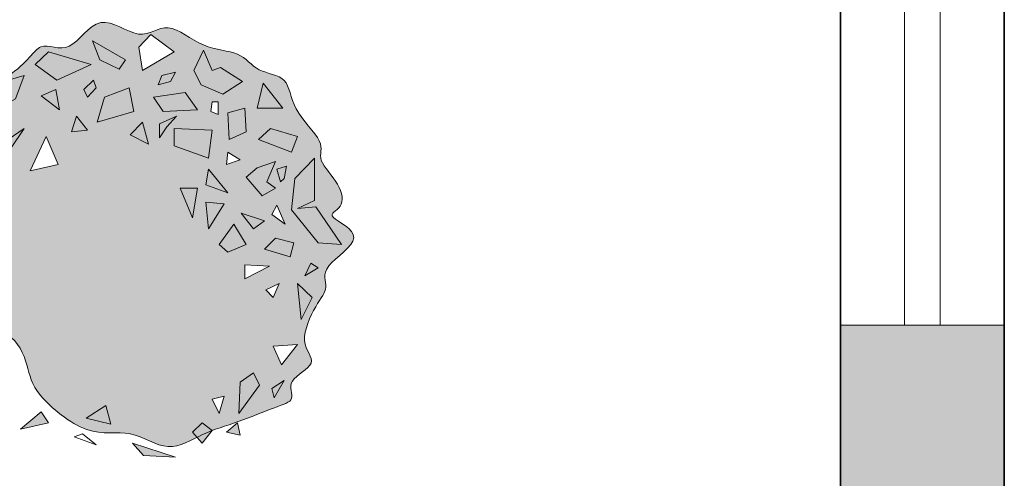
# Model space of a CAD drawing. Units: metres. Extents: x 4298.5 to 4325.2, y 2075 to 2095.8.
# Tile 14 of 35: x 4304.508 to 4305.891, y 2083.045 to 2083.689. Entities that reach past the tile are written whole.
import ezdxf

# ---------------------------------------------------------------- set-up
doc = ezdxf.new("R2010")
doc.units = ezdxf.units.M
for name, color, linetype, lineweight in [('A-ANNO-DIMS', 2, 'Continuous', 18), ('A-GLAZ', 4, 'Continuous', 18), ('A-WALL', 7, 'Continuous', 35), ('A-WALL-PATT', 252, 'Continuous', 13), ('L-PLNT', 94, 'Continuous', 13)]:
    doc.layers.add(name, color=color, linetype=linetype, lineweight=lineweight)
doc.layers.add('L-PLNT-PATT', color=116, linetype='Continuous', lineweight=13, true_color=0x13823e)
doc.styles.get("Standard").update_dxf_attribs({"font": 'arial.ttf'})
doc.dimstyles.get("Standard").update_dxf_attribs({"dimtxt": 0.18, "dimasz": 0.18, "dimexe": 0.18, "dimexo": 0.0625, "dimgap": 0.09, "dimtad": 0, "dimtih": 1, "dimtoh": 1, "dimdec": 4, "dimzin": 0, "dimdsep": 46, "dimtxsty": 'Standard', "dimcen": 0.09, "dimadec": 0, "dimazin": 0, "dimtfac": 1, "dimtdec": 4, "dimtofl": 0, "dimtmove": 0, "dimatfit": 3, "dimfxl": 1, "dimtolj": 1, "dimtzin": 0, "dimarcsym": 0})

# ---------------------------------------------------------------- blocks, each defined once
blk = doc.blocks.new('*U9')
for points in [[(1.237, 12.003), (0.562, 11.31), (0.764, 10.013), (2.519, 11.051)], [(-2.003, 11.656), (-1.598, 10.618), (-0.518, 10.099), (-0.181, 10.618), (-0.788, 10.964)], [(-4.432, 11.051), (-5.175, 10.359), (-3.96, 9.493), (-2.07, 10.359)], [(4.139, 11.137), (3.599, 10.013), (4.004, 9.234), (5.218, 8.715), (6.298, 9.407), (5.083, 10.186), (4.611, 10.013)], [(2.586, 9.926), (1.844, 9.753), (1.642, 9.234), (2.316, 9.407)], [(-5.782, 9.753), (-7.537, 9.234), (-8.009, 7.504), (-6.255, 8.455)], [(-1.935, 9.493), (-2.475, 8.974), (-2.273, 8.542), (-1.8, 9.061)], [(7.446, 9.32), (7.108, 7.936), (8.525, 7.936)], [(-4.837, 8.628), (-3.825, 7.85), (-4.027, 8.974)], [(0.022, 9.061), (-1.328, 8.542), (-1.733, 7.157), (0.292, 7.763)], [(1.372, 8.542), (3.126, 8.801), (3.801, 7.85), (1.912, 7.763)], [(4.611, 8.282), (4.544, 7.763), (4.949, 7.59), (4.949, 8.282)], [(6.433, 7.936), (5.488, 7.676), (5.556, 6.206), (6.501, 6.638)], [(-2.88, 7.504), (-3.15, 6.638), (-2.273, 6.725)], [(0.764, 7.157), (0.089, 6.465), (1.102, 5.946)], [(1.709, 6.292), (1.709, 7.071), (2.654, 7.504), (2.114, 6.898)], [(-5.782, 6.811), (-6.659, 6.206), (-6.524, 5.687)], [(2.519, 6.811), (2.519, 5.86), (4.409, 5.167), (4.611, 6.725)], [(7.851, 6.811), (7.176, 6.206), (8.998, 5.514), (9.335, 6.379)], [(-8.144, 6.033), (-9.359, 5.946), (-9.022, 4.735)], [(-4.567, 6.379), (-5.445, 4.475), (-3.892, 4.821)], [(5.488, 5.514), (5.421, 4.821), (6.163, 5.081)], [(8.12, 4.994), (7.108, 4.648), (6.501, 4.129), (7.378, 3.091), (8.12, 3.524), (7.648, 3.87)], [(10.28, 5.167), (9.2, 4.043), (8.998, 2.312), (10.482, 0.495), (11.765, 0.409), (10.348, 2.485), (9.335, 2.399), (10.28, 2.831)], [(4.409, 4.562), (4.274, 3.697), (5.488, 3.264)], [(8.728, 4.735), (8.188, 4.562), (8.39, 3.87), (8.593, 4.043)], [(-11.316, 1.793), (-9.831, 2.312), (-9.629, 3.437), (-10.439, 3.524)], [(3.531, 1.88), (2.856, 3.524), (3.801, 3.524)], [(-8.212, 3.091), (-8.482, 2.312), (-7.874, 2.572)], [(4.274, 2.745), (5.286, 2.658), (4.409, 1.274)], [(8.188, 2.572), (7.918, 2.053), (8.66, 1.534)], [(-6.997, 1.793), (-7.942, 1.534), (-7.469, 0.495)], [(7.513, 1.707), (6.906, 1.274), (6.231, 2.139)], [(5.826, 1.534), (5.016, 0.409), (5.488, -0.024), (6.501, 0.409)], [(-8.212, 0.409), (-9.426, 0.322), (-9.831, 0.841)], [(8.12, 0.755), (7.513, 0.149), (8.93, -0.283), (9.133, 0.495)], [(7.783, -0.803), (6.433, -1.495), (6.433, -0.716)], [(10.078, -0.629), (9.74, -1.322), (10.482, -0.889)], [(8.323, -1.754), (7.985, -2.533), (7.581, -2.1)], [(9.335, -1.754), (9.538, -3.744), (10.145, -2.533)], [(-10.034, -2.706), (-10.641, -3.312), (-10.439, -4.436), (-9.899, -3.485)], [(-8.279, -5.734), (-6.794, -5.302), (-6.997, -6.513)], [(9.335, -5.129), (8.458, -6.253), (7.985, -5.215)], [(6.096, -8.935), (6.163, -7.205), (6.906, -6.686), (7.243, -7.378)], [(8.053, -8.07), (8.593, -7.118), (7.918, -7.551)], [(5.286, -7.984), (4.611, -8.157), (5.016, -8.935)], [(-2.34, -9.195), (-1.26, -8.503), (-0.99, -9.541)], [(-4.837, -8.849), (-4.432, -9.454), (-5.985, -9.801)], [(4.071, -9.454), (3.531, -9.974), (4.071, -10.579), (4.611, -9.887)], [(6.028, -9.454), (5.421, -9.974), (6.163, -10.147)], [(-2.543, -10.06), (-3.015, -10.233), (-1.8, -10.666)], [(0.224, -10.579), (0.832, -11.272), (2.586, -11.358)]]:
    blk.add_lwpolyline(points, close=True)
blk = doc.blocks.new('WIN-760-GLASS')
for p, q in [((0, 0.76), (0, 0)), ((0.05, 0.76), (0.05, 0))]:
    blk.add_line(p, q)
blk = doc.blocks.new('*D47')
at = {"layer": 'A-ANNO-DIMS', "color": 0, "lineweight": -2, "transparency": 16777216}
for p, q in [((4300.4306, 2084.4956), (4300.4306, 2074.9896)), ((4322.8106, 2084.4956), (4322.8106, 2074.9896)), ((4300.6106, 2075.1696), (4311.2252, 2075.1696)), ((4322.6306, 2075.1696), (4312.016, 2075.1696))]:
    blk.add_line(p, q, dxfattribs=at)
at = {"layer": 'A-ANNO-DIMS', "color": 0, "transparency": 16777216}
for points in [[(4300.6106, 2075.1996), (4300.6106, 2075.1396), (4300.4306, 2075.1696)], [(4322.6306, 2075.1996), (4322.6306, 2075.1396), (4322.8106, 2075.1696)]]:
    blk.add_solid(points, dxfattribs=at)
at = {"layer": 'Defpoints', "color": 0, "transparency": 16777216}
for p in [(4300.4306, 2084.5581), (4322.8106, 2084.5581), (4322.8106, 2075.1696)]:
    blk.add_point(p, dxfattribs=at)
at = {"layer": 'A-ANNO-DIMS', "color": 0, "transparency": 16777216, "insert": (4311.6206, 2075.1696), "char_height": 0.18, "attachment_point": 5}
blk.add_mtext('\\A1;22.38', dxfattribs=at)
blk = doc.blocks.new('*D51')
at = {"layer": 'A-ANNO-DIMS', "color": 0, "lineweight": -2, "transparency": 16777216}
for p, q in [((4305.5981, 2084.5581), (4299.0921, 2084.5581)), ((4299.2721, 2084.3781), (4299.2721, 2082.375)), ((4299.2721, 2080.0081), (4299.2721, 2082.0111)), ((4305.5981, 2079.8281), (4299.0921, 2079.8281))]:
    blk.add_line(p, q, dxfattribs=at)
at = {"layer": 'A-ANNO-DIMS', "color": 0, "transparency": 16777216}
for points in [[(4299.2421, 2084.3781), (4299.3021, 2084.3781), (4299.2721, 2084.5581)], [(4299.2421, 2080.0081), (4299.3021, 2080.0081), (4299.2721, 2079.8281)]]:
    blk.add_solid(points, dxfattribs=at)
at = {"layer": 'Defpoints', "color": 0, "transparency": 16777216}
for p in [(4305.6606, 2084.5581), (4299.2721, 2079.8281), (4305.6606, 2079.8281)]:
    blk.add_point(p, dxfattribs=at)
at = {"layer": 'A-ANNO-DIMS', "color": 0, "transparency": 16777216, "insert": (4299.2721, 2082.1931), "char_height": 0.18, "attachment_point": 5}
blk.add_mtext('\\A1;4.73', dxfattribs=at)
blk = doc.blocks.new('*D56')
at = {"layer": 'A-ANNO-DIMS', "color": 0, "lineweight": -2, "transparency": 16777216}
for p, q in [((4305.8281, 2085.0581), (4299.0921, 2085.0581)), ((4299.2721, 2084.8781), (4299.2721, 2083.74)), ((4299.2721, 2082.2381), (4299.2721, 2083.3761)), ((4305.8281, 2082.0581), (4299.0921, 2082.0581))]:
    blk.add_line(p, q, dxfattribs=at)
at = {"layer": 'A-ANNO-DIMS', "color": 0, "transparency": 16777216}
for points in [[(4299.2421, 2084.8781), (4299.3021, 2084.8781), (4299.2721, 2085.0581)], [(4299.2421, 2082.2381), (4299.3021, 2082.2381), (4299.2721, 2082.0581)]]:
    blk.add_solid(points, dxfattribs=at)
at = {"layer": 'Defpoints', "color": 0, "transparency": 16777216}
for p in [(4299.2721, 2085.0581), (4305.8906, 2085.0581), (4305.8906, 2082.0581)]:
    blk.add_point(p, dxfattribs=at)
at = {"layer": 'A-ANNO-DIMS', "color": 0, "transparency": 16777216, "insert": (4299.2721, 2083.5581), "char_height": 0.18, "attachment_point": 5}
blk.add_mtext('\\A1;3', dxfattribs=at)

msp = doc.modelspace()

# ---------------------------------------------------------------- hatches: boundary and pattern name
at = {"layer": 'A-WALL-PATT'}
h = msp.add_hatch(color=256, dxfattribs=at)
h.dxf.hatch_style = 1
h.paths.add_polyline_path([(4308.7606, 2094.4781), (4308.1606, 2094.4781), (4307.4606, 2094.4781), (4307.4606, 2094.2481), (4308.2706, 2094.2481), (4308.2706, 2094.1281), (4308.3906, 2094.1281), (4308.3906, 2094.2481), (4308.7606, 2094.2481)])
h.paths.add_polyline_path([(4310.1206, 2094.4781), (4309.5206, 2094.4781), (4309.5206, 2094.2481), (4309.8906, 2094.2481), (4309.8906, 2092.2481), (4308.3906, 2092.2481), (4308.3906, 2093.4281), (4308.2706, 2093.4281), (4308.2706, 2092.0181), (4309.8906, 2092.0181), (4309.8906, 2087.0181), (4309.7706, 2087.0181), (4309.7706, 2086.7881), (4309.8906, 2086.7881), (4311.9406, 2086.7881), (4311.9406, 2087.0181), (4310.1206, 2087.0181), (4310.1206, 2089.0181), (4310.2406, 2089.0181), (4310.2406, 2089.1381), (4310.1206, 2089.1381), (4310.1206, 2092.0181), (4310.3078, 2092.0181), (4310.3078, 2092.2481), (4310.1206, 2092.2481)])
h.paths.add_polyline_path([(4311.7406, 2092.2481), (4311.0678, 2092.2481), (4311.0678, 2092.0181), (4311.7406, 2092.0181)], flags=17)
h.paths.add_polyline_path([(4313.1733, 2092.2481), (4312.5006, 2092.2481), (4312.5006, 2092.0181), (4313.1733, 2092.0181)])
h.paths.add_polyline_path([(4314.5378, 2092.2481), (4314.1206, 2092.2481), (4313.9333, 2092.2481), (4313.9333, 2092.0181), (4314.1206, 2092.0181), (4314.1206, 2087.0181), (4314.0006, 2087.0181), (4314.0006, 2086.7881), (4314.1206, 2086.7881), (4315.5718, 2086.7881), (4315.5718, 2087.0181), (4314.3506, 2087.0181), (4314.3506, 2092.0181), (4314.5378, 2092.0181)])
h.paths.add_polyline_path([(4315.9706, 2092.2481), (4315.2978, 2092.2481), (4315.2978, 2092.0181), (4315.9706, 2092.0181)])
h.paths.add_polyline_path([(4317.4033, 2092.2481), (4316.7306, 2092.2481), (4316.7306, 2092.0181), (4317.4033, 2092.0181)])
h.paths.add_polyline_path([(4318.9506, 2092.2481), (4318.3506, 2092.2481), (4318.1633, 2092.2481), (4318.1633, 2092.0181), (4318.3506, 2092.0181), (4318.3506, 2091.8981), (4318.5806, 2091.8981), (4318.5806, 2092.0181), (4318.9506, 2092.0181)])
h.paths.add_polyline_path([(4321.0106, 2092.2481), (4319.7106, 2092.2481), (4319.7106, 2092.0181), (4320.0806, 2092.0181), (4320.0806, 2090.0181), (4318.5806, 2090.0181), (4318.5806, 2091.1981), (4318.3506, 2091.1981), (4318.3506, 2090.0181), (4318.3506, 2087.0181), (4318.2306, 2087.0181), (4318.2306, 2086.7881), (4318.3506, 2086.7881), (4318.3506, 2086.3081), (4318.5806, 2086.3081), (4318.5806, 2089.7881), (4321.7806, 2089.7881), (4321.7806, 2090.0181), (4320.2006, 2090.0181), (4320.2006, 2092.0181), (4321.0106, 2092.0181)])
h.paths.add_polyline_path([(4322.8106, 2092.2481), (4321.7706, 2092.2481), (4321.7706, 2092.0181), (4322.5806, 2092.0181), (4322.5806, 2091.2831), (4322.8106, 2091.2831)])
h.paths.add_polyline_path([(4322.8106, 2090.5231), (4322.5806, 2090.5231), (4322.5806, 2089.7881), (4322.5806, 2089.5254), (4322.8106, 2089.5254), (4322.8106, 2090.0181)])
h.paths.add_polyline_path([(4322.8106, 2088.7654), (4322.5806, 2088.7654), (4322.5806, 2087.6681), (4322.8106, 2087.6681)])
h.paths.add_polyline_path([(4322.8106, 2086.9081), (4322.5806, 2086.9081), (4322.5806, 2085.8107), (4322.8106, 2085.8107)])
h.paths.add_polyline_path([(4322.8106, 2085.0507), (4322.5806, 2085.0507), (4322.5806, 2084.7881), (4318.5806, 2084.7881), (4318.5806, 2085.0581), (4318.5806, 2085.4081), (4318.3506, 2085.4081), (4318.3506, 2084.5581), (4318.3506, 2080.8581), (4318.4706, 2080.8581), (4318.4706, 2082.3281), (4319.2606, 2082.3281), (4319.2606, 2082.5581), (4318.5806, 2082.5581), (4318.5806, 2084.5581), (4320.0806, 2084.5581), (4320.0806, 2083.9381), (4320.3106, 2083.9381), (4320.3106, 2084.5581), (4322.8106, 2084.5581)])
h.paths.add_polyline_path([(4320.3106, 2083.1781), (4320.0806, 2083.1781), (4320.0806, 2082.5581), (4319.9606, 2082.5581), (4319.9606, 2082.3281), (4320.0806, 2082.3281), (4320.0806, 2081.5731), (4320.3106, 2081.5731)], flags=17)
h.paths.add_polyline_path([(4320.3106, 2080.8131), (4320.0806, 2080.8131), (4320.0806, 2080.0581), (4318.4286, 2080.0581), (4318.4286, 2079.8281), (4320.3106, 2079.8281)])
h.paths.add_polyline_path([(4317.3506, 2085.2881), (4316.5718, 2085.2881), (4316.5718, 2085.0581), (4317.3506, 2085.0581)])
h.paths.add_polyline_path([(4315.5718, 2085.2881), (4314.8434, 2085.2881), (4314.8434, 2085.0581), (4315.5718, 2085.0581)])
h.paths.add_polyline_path([(4313.8434, 2085.2881), (4312.9406, 2085.2881), (4312.9406, 2085.0581), (4313.8434, 2085.0581)])
h.paths.add_polyline_path([(4311.9406, 2085.2881), (4311.4406, 2085.2881), (4311.4406, 2085.0581), (4311.9406, 2085.0581)])
h.paths.add_polyline_path([(4317.3306, 2087.0181), (4316.5718, 2087.0181), (4316.5718, 2086.7881), (4317.3306, 2086.7881)])
h.paths.add_polyline_path([(4313.1006, 2089.1381), (4311.1406, 2089.1381), (4311.1406, 2089.0181), (4312.9806, 2089.0181), (4312.9806, 2087.0181), (4312.9406, 2087.0181), (4312.9406, 2086.7881), (4313.1006, 2086.7881), (4313.1006, 2087.0181)])
h.paths.add_polyline_path([(4307.5515, 2087.0181), (4305.8906, 2087.0181), (4305.8906, 2092.2481), (4305.8906, 2094.2481), (4306.7006, 2094.2481), (4306.7006, 2094.4781), (4305.6606, 2094.4781), (4305.6606, 2092.2481), (4305.2906, 2092.2481), (4305.2906, 2092.0181), (4305.6606, 2092.0181), (4305.6606, 2090.0181), (4304.1606, 2090.0181), (4304.1606, 2091.1981), (4304.0406, 2091.1981), (4304.0406, 2089.9081), (4301.5606, 2089.9081), (4301.5606, 2089.7881), (4304.0406, 2089.7881), (4305.6606, 2089.7881), (4305.6606, 2086.6381), (4305.8906, 2086.6381), (4305.8906, 2086.7881), (4307.5515, 2086.7881)])
h.paths.add_polyline_path([(4307.5515, 2085.2881), (4305.8906, 2085.2881), (4305.8906, 2085.4381), (4305.6606, 2085.4381), (4305.6606, 2084.7881), (4305.2906, 2084.7881), (4305.2906, 2084.5581), (4305.6606, 2084.5581), (4305.6606, 2084.02), (4305.8906, 2084.02), (4305.8906, 2084.5581), (4305.8906, 2085.0581), (4307.5515, 2085.0581)])
h.paths.add_polyline_path([(4310.2406, 2085.2881), (4308.5515, 2085.2881), (4308.5515, 2085.0581), (4310.2406, 2085.0581)])
h.paths.add_polyline_path([(4317.4286, 2080.0581), (4316.5718, 2080.0581), (4316.5718, 2079.8281), (4317.4286, 2079.8281)])
h.paths.add_polyline_path([(4315.5718, 2080.0581), (4314.8434, 2080.0581), (4314.8434, 2079.8281), (4315.5718, 2079.8281)])
h.paths.add_polyline_path([(4313.8434, 2080.0581), (4312.9406, 2080.0581), (4312.9406, 2079.8281), (4313.8434, 2079.8281)])
h.paths.add_polyline_path([(4311.9406, 2080.0581), (4311.4406, 2080.0581), (4311.4406, 2079.8281), (4311.9406, 2079.8281)])
h.paths.add_polyline_path([(4310.2406, 2080.0581), (4310.1206, 2080.0581), (4310.1206, 2084.0381), (4309.8906, 2084.0381), (4309.8906, 2080.0581), (4309.1606, 2080.0581), (4309.1606, 2079.8281), (4310.2406, 2079.8281)])
h.paths.add_polyline_path([(4308.1606, 2080.0581), (4307.5106, 2080.0581), (4307.5106, 2080.1781), (4307.3906, 2080.1781), (4307.3906, 2080.0581), (4305.8906, 2080.0581), (4305.8906, 2080.567), (4305.6606, 2080.567), (4305.6606, 2079.8281), (4308.1606, 2079.8281)])
h.paths.add_polyline_path([(4307.5106, 2081.9381), (4309.0906, 2081.9381), (4309.0906, 2082.0581), (4305.8906, 2082.0581), (4305.8906, 2083.26), (4305.6606, 2083.26), (4305.6606, 2081.327), (4305.8906, 2081.327), (4305.8906, 2081.9381), (4307.3906, 2081.9381), (4307.3906, 2080.8781), (4307.5106, 2080.8781)])
h.paths.add_polyline_path([(4304.5306, 2084.7881), (4302.7306, 2084.7881), (4302.7306, 2084.5581), (4304.5306, 2084.5581)])
h.paths.add_polyline_path([(4301.9706, 2084.7881), (4300.6606, 2084.7881), (4300.6606, 2085.0249), (4300.4306, 2085.0249), (4300.4306, 2084.5581), (4301.9706, 2084.5581)])
h.paths.add_polyline_path([(4300.6606, 2086.8843), (4300.4306, 2086.8843), (4300.4306, 2085.7849), (4300.6606, 2085.7849)])
h.paths.add_polyline_path([(4300.6606, 2089.1618), (4300.4306, 2089.1618), (4300.4306, 2087.6443), (4300.6606, 2087.6443)])
h.paths.add_polyline_path([(4300.6606, 2091.0212), (4300.4306, 2091.0212), (4300.4306, 2089.9218), (4300.6606, 2089.9218)])
h.paths.add_polyline_path([(4300.6606, 2092.0181), (4301.9706, 2092.0181), (4301.9706, 2092.2481), (4300.4306, 2092.2481), (4300.4306, 2091.7812), (4300.6606, 2091.7812)])
h.paths.add_polyline_path([(4304.5306, 2092.2481), (4302.7306, 2092.2481), (4302.7306, 2092.0181), (4304.0406, 2092.0181), (4304.0406, 2091.8981), (4304.1606, 2091.8981), (4304.1606, 2092.0181), (4304.5306, 2092.0181)], flags=17)
at = {"layer": 'L-PLNT-PATT'}
h = msp.add_hatch(color=256, dxfattribs=at)
h.dxf.hatch_style = 1
edge = h.paths.add_edge_path()
edge.add_spline(control_points=[(4304.7568, 2083.1024), (4304.7594, 2083.1037), (4304.778, 2083.1131), (4304.8138, 2083.1228), (4304.8683, 2083.1461), (4304.8977, 2083.1537), (4304.8789, 2083.1822), (4304.9315, 2083.2063), (4304.8978, 2083.2327), (4304.9248, 2083.2924), (4304.9435, 2083.3119), (4304.9269, 2083.3404), (4305.0011, 2083.3852), (4304.9312, 2083.4148), (4304.9639, 2083.4224), (4304.9599, 2083.4576), (4304.9218, 2083.4942), (4304.9404, 2083.5135), (4304.8873, 2083.5645), (4304.8873, 2083.6106), (4304.8395, 2083.6139), (4304.819, 2083.6458), (4304.7658, 2083.6458), (4304.7135, 2083.6912), (4304.6787, 2083.6541), (4304.618, 2083.7049), (4304.5781, 2083.6349), (4304.5335, 2083.6648), (4304.5192, 2083.6255), (4304.4789, 2083.6024), (4304.4725, 2083.5985)], knot_values=[0.818571, 0.818571, 0.818571, 0.818571, 0.97924, 1.97924, 2.97924, 3.97924, 4.97924, 5.97924, 6.97924, 7.97924, 8.97924, 9.97924, 10.97924, 11.97924, 12.97924, 13.97924, 14.97924, 15.97924, 16.97924, 17.97924, 18.97924, 19.97924, 20.97924, 21.97924, 22.97924, 23.97924, 24.97924, 25.97924, 26.97924, 27.16067, 27.16067, 27.16067, 27.16067], degree=3, periodic=0)
edge.add_line((4304.4725, 2083.5985), (4304.5138, 2083.6107))
edge.add_line((4304.5138, 2083.6107), (4304.5018, 2083.5777))
edge.add_line((4304.5018, 2083.5777), (4304.4572, 2083.5536))
edge.add_line((4304.4572, 2083.5536), (4304.4689, 2083.5961))
edge.add_spline(control_points=[(4304.4689, 2083.5961), (4304.4462, 2083.5815), (4304.4229, 2083.5605), (4304.4256, 2083.5161)], knot_values=[0.141368, 0.141368, 0.141368, 0.141368, 0.783694, 0.783694, 0.783694, 0.783694], degree=3, periodic=0)
edge.add_spline(control_points=[(4304.4256, 2083.5161), (4304.4296, 2083.5159), (4304.4339, 2083.5155), (4304.4384, 2083.5151)], knot_values=[40.901028, 40.901028, 40.901028, 40.901028, 41, 41, 41, 41], degree=3, periodic=0)
edge.add_line((4304.4384, 2083.5151), (4304.4538, 2083.5162))
edge.add_line((4304.4538, 2083.5162), (4304.4315, 2083.4832))
edge.add_line((4304.4315, 2083.4832), (4304.423, 2083.514))
edge.add_line((4304.423, 2083.514), (4304.4258, 2083.5142))
edge.add_spline(control_points=[(4304.4258, 2083.5142), (4304.4257, 2083.5148), (4304.4257, 2083.5155), (4304.4256, 2083.5161)], knot_values=[0.13204, 0.13204, 0.13204, 0.13204, 0.141368, 0.141368, 0.141368, 0.141368], degree=3, periodic=0)
edge.add_spline(control_points=[(4304.4256, 2083.5161), (4304.3894, 2083.5185), (4304.3578, 2083.5086), (4304.3058, 2083.5506), (4304.3729, 2083.4481), (4304.3752, 2083.4212), (4304.3759, 2083.4137)], knot_values=[37.439141, 37.439141, 37.439141, 37.439141, 38.340169, 39.340169, 40.340169, 40.901028, 40.901028, 40.901028, 40.901028], degree=3, periodic=0)
edge.add_line((4304.3759, 2083.4137), (4304.3955, 2083.4525))
edge.add_line((4304.3955, 2083.4525), (4304.4161, 2083.4502))
edge.add_line((4304.4161, 2083.4502), (4304.411, 2083.4217))
edge.add_line((4304.411, 2083.4217), (4304.3763, 2083.4096))
edge.add_spline(control_points=[(4304.3763, 2083.4096), (4304.3768, 2083.4056), (4304.3799, 2083.3921), (4304.4212, 2083.3711), (4304.3998, 2083.2738), (4304.432, 2083.255), (4304.4983, 2083.255), (4304.521, 2083.2013), (4304.5245, 2083.1658), (4304.6055, 2083.0997), (4304.6638, 2083.1165), (4304.7142, 2083.0796), (4304.7433, 2083.0956), (4304.7568, 2083.1024)], knot_values=[27.16067, 27.16067, 27.16067, 27.16067, 27.490087, 28.490087, 29.490087, 30.490087, 31.490087, 32.490087, 33.490087, 34.490087, 35.490087, 36.490087, 37.329418, 37.329418, 37.329418, 37.329418], degree=3, periodic=0)
edge.add_line((4304.7568, 2083.1024), (4304.7504, 2083.1096))
edge.add_line((4304.7504, 2083.1096), (4304.7641, 2083.1228))
edge.add_line((4304.7641, 2083.1228), (4304.7778, 2083.1118))
h.paths.add_polyline_path([(4304.7332, 2083.4525), (4304.7572, 2083.4525), (4304.7504, 2083.4107)], flags=16)
h.paths.add_polyline_path([(4304.7692, 2083.4327), (4304.7949, 2083.4305), (4304.7727, 2083.3953)], flags=16)
h.paths.add_polyline_path([(4304.5618, 2083.4854), (4304.5224, 2083.4766), (4304.5447, 2083.525)], flags=16)
h.paths.add_polyline_path([(4304.6887, 2083.514), (4304.6629, 2083.5272), (4304.6801, 2083.5447)], flags=16)
h.paths.add_polyline_path([(4304.7692, 2083.4569), (4304.7727, 2083.4788), (4304.8001, 2083.4459)], flags=16)
h.paths.add_polyline_path([(4304.7881, 2083.3733), (4304.8087, 2083.4019), (4304.8258, 2083.3733), (4304.8001, 2083.3623)], flags=16)
h.paths.add_polyline_path([(4304.7247, 2083.5118), (4304.7247, 2083.5359), (4304.7778, 2083.5338), (4304.7727, 2083.4942)], flags=16)
h.paths.add_polyline_path([(4304.7041, 2083.5228), (4304.7041, 2083.5426), (4304.7281, 2083.5536), (4304.7144, 2083.5382)], flags=16)
h.paths.add_polyline_path([(4304.6029, 2083.5338), (4304.5807, 2083.5316), (4304.5875, 2083.5536)], flags=16)
h.paths.add_polyline_path([(4304.6167, 2083.5447), (4304.6269, 2083.5799), (4304.6612, 2083.5931), (4304.6681, 2083.5601)], flags=16)
h.paths.add_polyline_path([(4304.4829, 2083.4085), (4304.471, 2083.3755), (4304.4589, 2083.4019)], flags=16)
h.paths.add_polyline_path([(4304.8189, 2083.4173), (4304.8515, 2083.4063), (4304.8361, 2083.3953)], flags=16)
h.paths.add_polyline_path([(4304.7984, 2083.4854), (4304.8001, 2083.503), (4304.8172, 2083.492)], flags=16)
h.paths.add_polyline_path([(4304.7092, 2083.5601), (4304.6955, 2083.5799), (4304.7401, 2083.5865), (4304.7572, 2083.5623)], flags=16)
h.paths.add_polyline_path([(4304.8241, 2083.3448), (4304.8584, 2083.3426), (4304.8241, 2083.325)], flags=16)
h.paths.add_polyline_path([(4304.4607, 2083.4283), (4304.4452, 2083.4217), (4304.4521, 2083.4415)], flags=16)
h.paths.add_polyline_path([(4304.5635, 2083.5623), (4304.5378, 2083.5821), (4304.5584, 2083.5909)], flags=16)
h.paths.add_polyline_path([(4304.495, 2083.5074), (4304.4915, 2083.5206), (4304.5138, 2083.5359)], flags=16)
h.paths.add_polyline_path([(4304.6029, 2083.5799), (4304.5978, 2083.5909), (4304.6115, 2083.6041), (4304.615, 2083.5931)], flags=16)
h.paths.add_polyline_path([(4304.8258, 2083.4678), (4304.8412, 2083.481), (4304.8669, 2083.4898), (4304.8549, 2083.4612), (4304.8669, 2083.4525), (4304.8481, 2083.4415)], flags=16)
h.paths.add_polyline_path([(4304.4521, 2083.3733), (4304.4212, 2083.3711), (4304.411, 2083.3843)], flags=16)
h.paths.add_polyline_path([(4304.8018, 2083.5206), (4304.8001, 2083.5579), (4304.8241, 2083.5645), (4304.8258, 2083.5316)], flags=16)
h.paths.add_polyline_path([(4304.8515, 2083.3667), (4304.8669, 2083.3821), (4304.8926, 2083.3755), (4304.8875, 2083.3558)], flags=16)
h.paths.add_polyline_path([(4304.7761, 2083.5601), (4304.7778, 2083.5733), (4304.7864, 2083.5733), (4304.7864, 2083.5557)], flags=16)
h.paths.add_polyline_path([(4304.7024, 2083.5975), (4304.7075, 2083.6107), (4304.7264, 2083.6151), (4304.7195, 2083.6019)], flags=16)
h.paths.add_polyline_path([(4304.8618, 2083.4151), (4304.8686, 2083.4283), (4304.8806, 2083.4019)], flags=16)
h.paths.add_polyline_path([(4304.8532, 2083.3096), (4304.8721, 2083.3184), (4304.8635, 2083.2986)], flags=16)
h.paths.add_polyline_path([(4304.6475, 2083.6195), (4304.6201, 2083.6326), (4304.6098, 2083.659), (4304.6407, 2083.6414), (4304.6561, 2083.6326)], flags=16)
h.paths.add_polyline_path([(4304.6801, 2083.6173), (4304.6749, 2083.6502), (4304.6921, 2083.6678), (4304.7247, 2083.6436)], flags=16)
h.paths.add_polyline_path([(4304.5601, 2083.6041), (4304.5292, 2083.6261), (4304.5481, 2083.6436), (4304.6081, 2083.6261)], flags=16)
h.paths.add_polyline_path([(4304.8429, 2083.5206), (4304.8601, 2083.5359), (4304.8978, 2083.525), (4304.8892, 2083.503)], flags=16)
h.paths.add_polyline_path([(4304.7624, 2083.5975), (4304.7521, 2083.6173), (4304.7658, 2083.6458), (4304.7778, 2083.6173), (4304.7898, 2083.6217), (4304.8206, 2083.6019), (4304.7932, 2083.5843)], flags=16)
h.paths.add_polyline_path([(4304.8738, 2083.4612), (4304.8686, 2083.4788), (4304.8824, 2083.4832), (4304.8789, 2083.4656)], flags=16)
h.paths.add_polyline_path([(4304.8892, 2083.4217), (4304.8944, 2083.4656), (4304.9218, 2083.4942), (4304.9218, 2083.4349), (4304.8978, 2083.4239), (4304.9235, 2083.4261), (4304.9595, 2083.3733), (4304.9269, 2083.3755)], flags=16)
h.paths.add_polyline_path([(4304.6287, 2083.147), (4304.6355, 2083.1206), (4304.6012, 2083.1294)], flags=16)
h.paths.add_polyline_path([(4304.8412, 2083.5645), (4304.8498, 2083.5997), (4304.8772, 2083.5645)], flags=16)
h.paths.add_polyline_path([(4304.8978, 2083.3184), (4304.9184, 2083.2986), (4304.9029, 2083.2679)], flags=16)
h.paths.add_polyline_path([(4304.9081, 2083.3294), (4304.9167, 2083.347), (4304.9269, 2083.3404)], flags=16)
h.paths.add_polyline_path([(4304.7778, 2083.1558), (4304.7949, 2083.1602), (4304.7881, 2083.136)], flags=16)
h.paths.add_polyline_path([(4304.8635, 2083.2305), (4304.8978, 2083.2327), (4304.8755, 2083.2041)], flags=16)
h.paths.add_polyline_path([(4304.8172, 2083.1799), (4304.8361, 2083.1931), (4304.8446, 2083.1755), (4304.8155, 2083.136)], flags=16)
h.paths.add_polyline_path([(4304.8618, 2083.1712), (4304.8789, 2083.1822), (4304.8652, 2083.158)], flags=16)
h = msp.add_hatch(color=256, dxfattribs=at)
h.dxf.hatch_style = 1
h.paths.add_polyline_path([(4304.7727, 2083.4942), (4304.7778, 2083.5338), (4304.7247, 2083.5359), (4304.7247, 2083.5118)])
h.paths.add_polyline_path([(4304.8189, 2083.4173), (4304.8361, 2083.3953), (4304.8515, 2083.4063)])
h.paths.add_polyline_path([(4304.8001, 2083.5579), (4304.8018, 2083.5206), (4304.8258, 2083.5316), (4304.8241, 2083.5645)])
h.paths.add_polyline_path([(4304.8206, 2083.6019), (4304.7898, 2083.6217), (4304.7778, 2083.6173), (4304.7658, 2083.6458), (4304.7521, 2083.6173), (4304.7624, 2083.5975), (4304.7932, 2083.5843)])
h.paths.add_polyline_path([(4304.6664, 2083.0942), (4304.6818, 2083.0766), (4304.7264, 2083.0745)])
h.paths.add_polyline_path([(4304.6475, 2083.6195), (4304.6561, 2083.6326), (4304.6407, 2083.6414), (4304.6098, 2083.659), (4304.6201, 2083.6326)])
h.paths.add_polyline_path([(4304.5481, 2083.6436), (4304.5292, 2083.6261), (4304.5601, 2083.6041), (4304.6081, 2083.6261)])
h.paths.add_polyline_path([(4304.6269, 2083.5799), (4304.6167, 2083.5447), (4304.6681, 2083.5601), (4304.6612, 2083.5931)])
h.paths.add_polyline_path([(4304.615, 2083.5931), (4304.6115, 2083.6041), (4304.5978, 2083.5909), (4304.6029, 2083.5799)])
h.paths.add_polyline_path([(4304.5875, 2083.5536), (4304.5807, 2083.5316), (4304.6029, 2083.5338)])
h.paths.add_polyline_path([(4304.5635, 2083.5623), (4304.5584, 2083.5909), (4304.5378, 2083.5821)])
h.paths.add_polyline_path([(4304.4692, 2083.5975), (4304.4572, 2083.5536), (4304.5018, 2083.5777), (4304.5138, 2083.6107)])
h.paths.add_polyline_path([(4304.5138, 2083.5359), (4304.4915, 2083.5206), (4304.495, 2083.5074)])
h.paths.add_polyline_path([(4304.423, 2083.514), (4304.4315, 2083.4832), (4304.4538, 2083.5162)])
h.paths.add_polyline_path([(4304.3732, 2083.4085), (4304.411, 2083.4217), (4304.4161, 2083.4502), (4304.3955, 2083.4525)])
h.paths.add_polyline_path([(4304.4829, 2083.4085), (4304.4589, 2083.4019), (4304.471, 2083.3755)])
h.paths.add_polyline_path([(4304.4092, 2083.2744), (4304.4058, 2083.2942), (4304.3904, 2083.2788), (4304.3955, 2083.2503)])
h.paths.add_polyline_path([(4304.4881, 2083.2283), (4304.4504, 2083.2173), (4304.4829, 2083.1975)])
h.paths.add_polyline_path([(4304.5087, 2083.114), (4304.5481, 2083.1228), (4304.5378, 2083.1382)])
h.paths.add_polyline_path([(4304.6287, 2083.147), (4304.6012, 2083.1294), (4304.6355, 2083.1206)])
h.paths.add_polyline_path([(4304.7641, 2083.1228), (4304.7504, 2083.1096), (4304.7641, 2083.0942), (4304.7778, 2083.1118)])
h.paths.add_polyline_path([(4304.8446, 2083.1755), (4304.8361, 2083.1931), (4304.8172, 2083.1799), (4304.8155, 2083.136)])
h.paths.add_polyline_path([(4304.8138, 2083.1228), (4304.7984, 2083.1096), (4304.8172, 2083.1052)])
h.paths.add_polyline_path([(4304.8618, 2083.1712), (4304.8652, 2083.158), (4304.8789, 2083.1822)])
h.paths.add_polyline_path([(4304.9029, 2083.2679), (4304.9184, 2083.2986), (4304.8978, 2083.3184)])
h.paths.add_polyline_path([(4304.7881, 2083.3733), (4304.8001, 2083.3623), (4304.8258, 2083.3733), (4304.8087, 2083.4019)])
h.paths.add_polyline_path([(4304.9269, 2083.3755), (4304.9595, 2083.3733), (4304.9235, 2083.4261), (4304.8978, 2083.4239), (4304.9218, 2083.4349), (4304.9218, 2083.4942), (4304.8944, 2083.4656), (4304.8892, 2083.4217)])
h.paths.add_polyline_path([(4304.8669, 2083.3821), (4304.8515, 2083.3667), (4304.8875, 2083.3558), (4304.8926, 2083.3755)])
h.paths.add_polyline_path([(4304.9269, 2083.3404), (4304.9167, 2083.347), (4304.9081, 2083.3294)])
h.paths.add_polyline_path([(4304.8669, 2083.4898), (4304.8412, 2083.481), (4304.8258, 2083.4678), (4304.8481, 2083.4415), (4304.8669, 2083.4525), (4304.8549, 2083.4612)])
h.paths.add_polyline_path([(4304.8686, 2083.4788), (4304.8738, 2083.4612), (4304.8789, 2083.4656), (4304.8824, 2083.4832)])
h.paths.add_polyline_path([(4304.8892, 2083.503), (4304.8978, 2083.525), (4304.8601, 2083.5359), (4304.8429, 2083.5206)])
h.paths.add_polyline_path([(4304.8001, 2083.4459), (4304.7727, 2083.4788), (4304.7692, 2083.4569)])
h.paths.add_polyline_path([(4304.7572, 2083.4525), (4304.7332, 2083.4525), (4304.7504, 2083.4107)])
h.paths.add_polyline_path([(4304.7949, 2083.4305), (4304.7692, 2083.4327), (4304.7727, 2083.3953)])
h.paths.add_polyline_path([(4304.7572, 2083.5623), (4304.7401, 2083.5865), (4304.6955, 2083.5799), (4304.7092, 2083.5601)])
h.paths.add_polyline_path([(4304.7144, 2083.5382), (4304.7281, 2083.5536), (4304.7041, 2083.5426), (4304.7041, 2083.5228)])
h.paths.add_polyline_path([(4304.6801, 2083.5447), (4304.6629, 2083.5272), (4304.6887, 2083.514)])
h.paths.add_polyline_path([(4304.7195, 2083.6019), (4304.7264, 2083.6151), (4304.7075, 2083.6107), (4304.7024, 2083.5975)])
h.paths.add_polyline_path([(4304.8498, 2083.5997), (4304.8412, 2083.5645), (4304.8772, 2083.5645)])

# ---------------------------------------------------------------- linework, layer by layer
at = {"layer": 'A-GLAZ'}
msp.add_line((4305.6606, 2083.26), (4305.8906, 2083.26), dxfattribs=at)
at = {"layer": 'A-WALL'}
for p, q in [((4305.6606, 2084.5581), (4305.6606, 2079.8281)), ((4305.8906, 2084.5581), (4305.8906, 2082.0581))]:
    msp.add_line(p, q, dxfattribs=at)
at = {"layer": 'L-PLNT'}
msp.add_open_spline([(4304.4315, 2083.4832), (4304.4074, 2083.5697), (4304.5138, 2083.6107), (4304.5335, 2083.6648), (4304.5781, 2083.6349), (4304.618, 2083.7049), (4304.6787, 2083.6541), (4304.7135, 2083.6912), (4304.7658, 2083.6458), (4304.819, 2083.6458), (4304.8395, 2083.6139), (4304.8873, 2083.6106), (4304.8873, 2083.5645), (4304.9404, 2083.5135), (4304.9218, 2083.4942), (4304.9599, 2083.4576), (4304.9639, 2083.4224), (4304.9312, 2083.4148), (4305.0011, 2083.3852), (4304.9269, 2083.3404), (4304.9435, 2083.3119), (4304.9248, 2083.2924), (4304.8978, 2083.2327), (4304.9315, 2083.2063), (4304.8789, 2083.1822), (4304.8977, 2083.1537), (4304.8683, 2083.1461), (4304.8138, 2083.1228), (4304.7641, 2083.1093), (4304.717, 2083.0775), (4304.6638, 2083.1165), (4304.6055, 2083.0997), (4304.5245, 2083.1658), (4304.521, 2083.2013), (4304.4983, 2083.255), (4304.432, 2083.255), (4304.3998, 2083.2738), (4304.4212, 2083.3711), (4304.368, 2083.3981), (4304.3844, 2083.4305), (4304.3058, 2083.5506), (4304.3596, 2083.5072), (4304.3927, 2083.5196), (4304.4384, 2083.5151)], degree=3, dxfattribs=at)

# ---------------------------------------------------------------- block references
at = {"layer": 'A-GLAZ', "rotation": 180}
msp.add_blockref('WIN-760-GLASS', (4305.8006, 2084.02), dxfattribs=at)
at = {"layer": 'L-PLNT', "xscale": 0.0254, "yscale": 0.0254, "zscale": 0.0254}
msp.add_blockref('*U9', (4304.6607, 2083.363), dxfattribs=at)

# ---------------------------------------------------------------- dimensions: what is measured, and where the dimension line sits
at = {"layer": 'A-ANNO-DIMS'}
for base, p1, p2, override, picture, middle in [((4299.2721, 2085.0581), (4305.8906, 2082.0581), (4305.8906, 2085.0581), {"dimdec": 0, "dimlfac": 1, "dimrnd": 0, "dimzin": 0, "dimdsep": 46, "dimlunit": 2}, '*D56', (4299.2721, 2083.5581)), ((4299.2721, 2079.8281), (4305.6606, 2084.5581), (4305.6606, 2079.8281), {"dimdec": 2, "dimlfac": 1, "dimrnd": 0, "dimzin": 0, "dimdsep": 46, "dimlunit": 2}, '*D51', (4299.2721, 2082.1931))]:
    dim = msp.add_linear_dim(base=base, p1=p1, p2=p2, angle=90, dimstyle='Standard', override=override, dxfattribs=at)
    dim.commit()
    dim.dimension.update_dxf_attribs({"geometry": picture, "text_midpoint": middle})
dim = msp.add_linear_dim(base=(4322.8106, 2075.1696), p1=(4300.4306, 2084.5581), p2=(4322.8106, 2084.5581), dimstyle='Standard', override={"dimdec": 2, "dimlfac": 1, "dimrnd": 0, "dimzin": 0, "dimdsep": 46, "dimlunit": 2}, dxfattribs=at)
dim.commit()
dim.dimension.update_dxf_attribs({"geometry": '*D47', "text_midpoint": (4311.6206, 2075.1696)})

doc.saveas('drawing.dxf')
